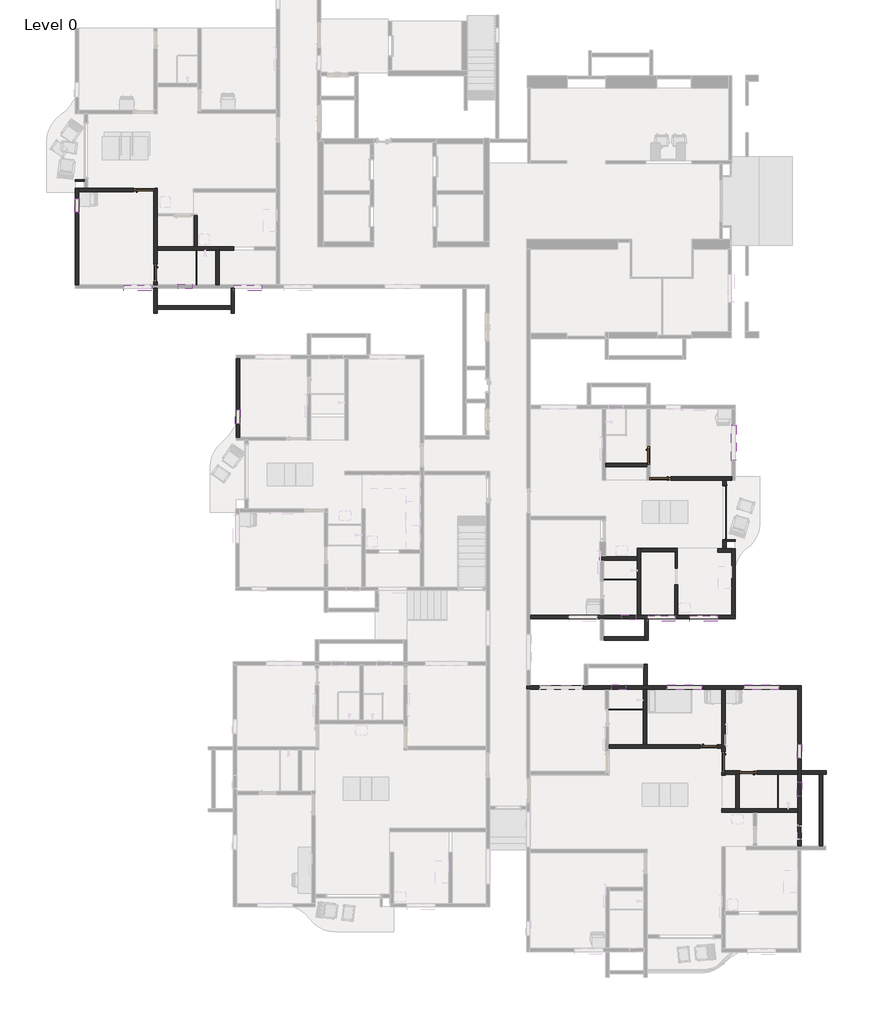
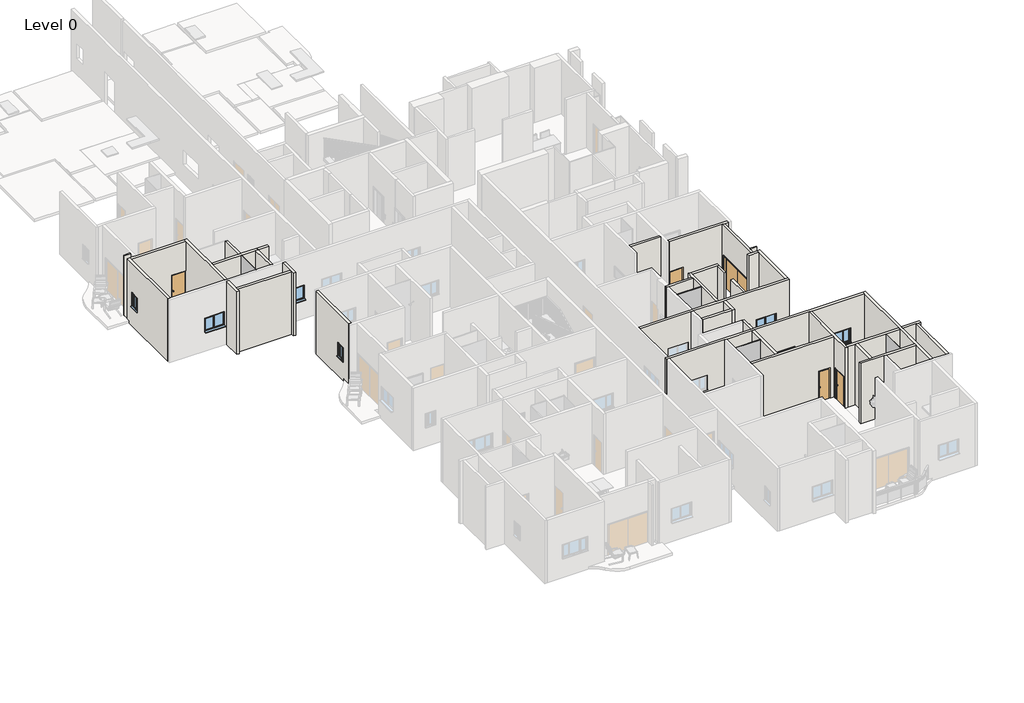
# One storey, part 3 of 14: 35 walls, 14 windows, 8 doors, 4 plates.
"""IFC4 building model written with IfcOpenShell, lengths in millimetres."""

from ifc_helpers import new_model, si_unit, frame, origin, origin_with_axes, place, context, project, spatial, polyline, outline, extrude, faceted_brep, transform, mapped, element, save
from components import doors_concept_intdbl_8_5090a96f, doors_extsgl_flush_d2_fac1298c, doors_extsgl_flush_d2_5e0ff3e2, doors_extsgl_flush_d3_352cde1d, doors_extsgl_flush_d3_ba5ff989, system_panel_glazed_533a1375, system_panel_glazed_d137d5b4, system_panel_glazed_d14c18e3, system_panel_glazed_5123bacf, windows_concept_plain_dbl_4_d1e2e333, windows_sgl_plain_2_be143095, windows_tpl_variable_casement_2_47b04551, windows_tpl_variable_casement_5_ffad3fa3

model = new_model("IFC4")

# Units and contexts
model_context = context("Model", 3, world=origin())
ifc_project = project(units=[si_unit("LENGTHUNIT", "METRE", prefix="MILLI")], contexts=[model_context])

# Site, building, storey
site = spatial("IfcSite", under=ifc_project)
building = spatial("IfcBuilding", under=site)
storey = spatial("IfcBuildingStorey", under=building, Name="Level 0", Elevation=0.0)

# Doors
placement = place(None, origin())
doors_concept_intdbl_8_shape = doors_concept_intdbl_8_5090a96f(model_context)
element("IfcDoor", 1, ObjectType="Doors_Concept_IntDbl : 8'", at=placement, inside=storey, context=model_context, shape_type="MappedRepresentation", body=[
    mapped(doors_concept_intdbl_8_shape, transform((-11246.4933798, 29202.1106683, 0.0), x_axis=(0.0, -1.0, 0.0), y_axis=(1.0, 0.0, 0.0), z_axis=(0.0, 0.0, 1.0))),
])
doors_extsgl_flush_d2_shape = doors_extsgl_flush_d2_fac1298c(model_context)
element("IfcDoor", 2, ObjectType="Doors_ExtSgl_Flush : D2", at=placement, inside=storey, context=model_context, shape_type="MappedRepresentation", body=[
    mapped(doors_extsgl_flush_d2_shape, transform((-11299.3465173, 18242.0106683, 0.0), x_axis=(0.0, -1.0, 0.0), y_axis=(1.0, 0.0, 0.0), z_axis=(0.0, 0.0, 1.0))),
])
doors_extsgl_flush_d2_2_shape = doors_extsgl_flush_d2_5e0ff3e2(model_context)
element("IfcDoor", 3, ObjectType="Doors_ExtSgl_Flush : D2", at=placement, inside=storey, context=model_context, shape_type="MappedRepresentation", body=[
    mapped(doors_extsgl_flush_d2_2_shape, transform((-14088.8486976, 30700.7106683, 0.0), x_axis=(-1.0, 0.0, 0.0), y_axis=(0.0, -1.0, 0.0), z_axis=(0.0, 0.0, 1.0))),
])
element("IfcDoor", 4, ObjectType="Doors_ExtSgl_Flush : D2", at=placement, inside=storey, context=model_context, shape_type="MappedRepresentation", body=[
    mapped(doors_extsgl_flush_d2_2_shape, transform((-36777.1839022, 43403.2998557, 0.0), x_axis=(1.0, 0.0, 0.0), y_axis=(0.0, 1.0, 0.0), z_axis=(0.0, 0.0, 1.0))),
])
doors_extsgl_flush_d3_shape = doors_extsgl_flush_d3_352cde1d(model_context)
element("IfcDoor", 5, ObjectType="Doors_ExtSgl_Flush : D3", at=placement, inside=storey, context=model_context, shape_type="MappedRepresentation", body=[
    mapped(doors_extsgl_flush_d3_shape, transform((-11947.1481173, 18921.5114683, 0.0), x_axis=(1.0, 0.0, 0.0), y_axis=(0.0, 1.0, 0.0), z_axis=(0.0, 0.0, 1.0))),
])
element("IfcDoor", 6, ObjectType="Doors_ExtSgl_Flush : D3", at=placement, inside=storey, context=model_context, shape_type="MappedRepresentation", body=[
    mapped(doors_extsgl_flush_d3_shape, transform((-10211.6953327, 17778.5114683, 0.0), x_axis=(-1.0, 0.0, 0.0), y_axis=(0.0, -1.0, 0.0), z_axis=(0.0, 0.0, 1.0))),
])
element("IfcDoor", 7, ObjectType="Doors_ExtSgl_Flush : D3", at=placement, inside=storey, context=model_context, shape_type="MappedRepresentation", body=[
    mapped(doors_extsgl_flush_d3_shape, transform((-36281.7823022, 39752.8962471, 0.0), x_axis=(0.0, -1.0, 0.0), y_axis=(1.0, 0.0, 0.0), z_axis=(0.0, 0.0, 1.0))),
])
doors_extsgl_flush_d3_2_shape = doors_extsgl_flush_d3_ba5ff989(model_context)
element("IfcDoor", 8, ObjectType="Doors_ExtSgl_Flush : D3", at=placement, inside=storey, context=model_context, shape_type="MappedRepresentation", body=[
    mapped(doors_extsgl_flush_d3_2_shape, transform((-14596.8486976, 31716.7106683, 0.0), x_axis=(0.0, -1.0, 0.0), y_axis=(1.0, 0.0, 0.0), z_axis=(0.0, 0.0, 1.0))),
])

# Plates
system_panel_glazed_shape = system_panel_glazed_533a1375(model_context)
element("IfcPlate", 9, ObjectType="System Panel : Glazed", at=placement, inside=storey, context=model_context, shape_type="MappedRepresentation", body=[
    mapped(system_panel_glazed_shape, transform((-34528.7632652, 39996.9988514, 0.0), x_axis=(0.0, -1.0, 0.0), y_axis=(1.0, 0.0, 0.0), z_axis=(0.0, 0.0, 1.0))),
])
system_panel_glazed_2_shape = system_panel_glazed_d137d5b4(model_context)
element("IfcPlate", 10, ObjectType="System Panel : Glazed", at=placement, inside=storey, context=model_context, shape_type="MappedRepresentation", body=[
    mapped(system_panel_glazed_2_shape, transform((-8932.7419991, 16923.8396258, 0.0), x_axis=(0.0, -1.0, 0.0), y_axis=(1.0, 0.0, 0.0), z_axis=(0.0, 0.0, 1.0))),
])
system_panel_glazed_3_shape = system_panel_glazed_d14c18e3(model_context)
element("IfcPlate", 11, ObjectType="System Panel : Glazed", at=placement, inside=storey, context=model_context, shape_type="MappedRepresentation", body=[
    mapped(system_panel_glazed_3_shape, transform((-15581.2639165, 20578.9122683, 0.0), x_axis=(-1.0, 0.0, 0.0), y_axis=(0.0, -1.0, 0.0), z_axis=(0.0, 0.0, 1.0))),
])
system_panel_glazed_4_shape = system_panel_glazed_5123bacf(model_context)
element("IfcPlate", 12, ObjectType="System Panel : Glazed", at=placement, inside=storey, context=model_context, shape_type="MappedRepresentation", body=[
    mapped(system_panel_glazed_4_shape, transform((-15827.0456172, 26227.359605, 0.0), x_axis=(1.0, 0.0, 0.0), y_axis=(0.0, 1.0, 0.0), z_axis=(0.0, 0.0, 1.0))),
])

# Walls
element("IfcWall", 13, ObjectType="W1", at=placement, inside=storey, context=model_context, shape_type="Brep", body=[
    faceted_brep([(-8039.9933343, 21594.9122683, 0.0), (-8039.9933343, 21442.5122683, 0.0), (-8039.9933343, 17854.7114683, 0.0), (-8039.9933343, 17702.3114683, 0.0), (-8039.9933343, 16175.8530766, 0.0), (-8039.9933343, 16023.4530766, 0.0), (-8039.9933343, 14528.3736639, 0.0), (-8039.9933343, 14528.3736639, 4000.0), (-8039.9933343, 16023.4530766, 4000.0), (-8039.9933343, 16175.8530766, 4000.0), (-8039.9933343, 17702.3114683, 4000.0), (-8039.9933343, 17854.7114683, 4000.0), (-8039.9933343, 21442.5122683, 4000.0), (-8039.9933343, 21594.9122683, 4000.0), (-8039.9933343, 19020.6530766, 2110.0), (-8039.9933343, 18411.0530766, 2110.0), (-8039.9933343, 18411.0530766, 1200.0), (-8039.9933343, 19020.6530766, 1200.0), (-8039.9933343, 15442.7736639, 2738.9328), (-8039.9933343, 14833.1736639, 2738.9328), (-8039.9933343, 14833.1736639, 1828.9328), (-8039.9933343, 15442.7736639, 1828.9328), (-8039.9933343, 17344.2530766, 2738.9328), (-8039.9933343, 16734.6530766, 2738.9328), (-8039.9933343, 16734.6530766, 1828.9328), (-8039.9933343, 17344.2530766, 1828.9328), (-7887.5933343, 21594.9122683, 0.0), (-7887.5933343, 21594.9122683, 4000.0), (-7887.5933343, 17854.7114683, 4000.0), (-7887.5933343, 17702.3114683, 4000.0), (-7887.5933343, 14528.3736639, 4000.0), (-7887.5933343, 14528.3736639, 0.0), (-7887.5933343, 17702.3114683, 0.0), (-7887.5933343, 17854.7114683, 0.0), (-7887.5933343, 19020.6530766, 2110.0), (-7887.5933343, 19020.6530766, 1200.0), (-7887.5933343, 18411.0530766, 1200.0), (-7887.5933343, 18411.0530766, 2110.0), (-7887.5933343, 15442.7736639, 2738.9328), (-7887.5933343, 15442.7736639, 1828.9328), (-7887.5933343, 14833.1736639, 1828.9328), (-7887.5933343, 14833.1736639, 2738.9328), (-7887.5933343, 17344.2530766, 2738.9328), (-7887.5933343, 17344.2530766, 1828.9328), (-7887.5933343, 16734.6530766, 1828.9328), (-7887.5933343, 16734.6530766, 2738.9328)], [[[0, 1, 2, 3, 4, 5, 6, 7, 8, 9, 10, 11, 12, 13], [14, 15, 16, 17], [18, 19, 20, 21], [22, 23, 24, 25]], [[26, 27, 28, 29, 30, 31, 32, 33], [34, 35, 36, 37], [38, 39, 40, 41], [42, 43, 44, 45]], [[6, 5, 4, 3, 2, 1, 0, 26, 33, 32, 31]], [[13, 12, 11, 10, 9, 8, 7, 30, 29, 28, 27]], [[7, 6, 31, 30]], [[0, 13, 27, 26]], [[35, 34, 14, 17]], [[36, 35, 17, 16]], [[37, 36, 16, 15]], [[34, 37, 15, 14]], [[39, 38, 18, 21]], [[40, 39, 21, 20]], [[41, 40, 20, 19]], [[38, 41, 19, 18]], [[43, 42, 22, 25]], [[44, 43, 25, 24]], [[45, 44, 24, 23]], [[42, 45, 23, 22]]]),
])
element("IfcWall", 14, ObjectType="W1", at=placement, inside=storey, context=model_context, shape_type="Brep", body=[
    faceted_brep([(-8039.9933343, 21594.9122683, 0.0), (-14657.7537173, 21594.9122683, 0.0), (-14810.1537173, 21594.9122683, 0.0), (-17277.7094141, 21594.9122683, 0.0), (-17430.1094141, 21594.9122683, 0.0), (-19793.4917798, 21594.9122683, 0.0), (-19945.8917798, 21594.9122683, 0.0), (-19965.3949343, 21594.9122683, 0.0), (-19965.3949343, 21594.9122683, 4000.0), (-19945.8917798, 21594.9122683, 4000.0), (-19793.4917798, 21594.9122683, 4000.0), (-17430.1094141, 21594.9122683, 4000.0), (-17277.7094141, 21594.9122683, 4000.0), (-14810.1537173, 21594.9122683, 4000.0), (-14657.7537173, 21594.9122683, 4000.0), (-8039.9933343, 21594.9122683, 4000.0), (-19360.5094141, 21594.9122683, 2110.0), (-19360.5094141, 21594.9122683, 1200.0), (-17531.7094141, 21594.9122683, 1200.0), (-17531.7094141, 21594.9122683, 2110.0), (-13778.6501173, 21594.9122683, 2110.0), (-13778.6501173, 21594.9122683, 1200.0), (-12254.6501173, 21594.9122683, 1200.0), (-12254.6501173, 21594.9122683, 2110.0), (-10393.5699258, 21594.9122683, 2110.0), (-10393.5699258, 21594.9122683, 1200.0), (-8869.5699258, 21594.9122683, 1200.0), (-8869.5699258, 21594.9122683, 2110.0), (-16212.6741157, 21594.9122683, 2738.9328), (-16212.6741157, 21594.9122683, 1828.9328), (-15603.0741157, 21594.9122683, 1828.9328), (-15603.0741157, 21594.9122683, 2738.9328), (-8039.9933343, 21442.5122683, 0.0), (-8039.9933343, 21442.5122683, 4000.0), (-11223.1465173, 21442.5122683, 4000.0), (-11375.5465173, 21442.5122683, 4000.0), (-14670.4537173, 21442.5122683, 4000.0), (-14822.8537173, 21442.5122683, 4000.0), (-16339.6741157, 21442.5122683, 4000.0), (-16492.0741157, 21442.5122683, 4000.0), (-19812.9949343, 21442.5122683, 4000.0), (-19965.3949343, 21442.5122683, 4000.0), (-19965.3949343, 21442.5122683, 0.0), (-19812.9949343, 21442.5122683, 0.0), (-16492.0741157, 21442.5122683, 0.0), (-16339.6741157, 21442.5122683, 0.0), (-14822.8537173, 21442.5122683, 0.0), (-14670.4537173, 21442.5122683, 0.0), (-11375.5465173, 21442.5122683, 0.0), (-11223.1465173, 21442.5122683, 0.0), (-19360.5094141, 21442.5122683, 2110.0), (-17531.7094141, 21442.5122683, 2110.0), (-17531.7094141, 21442.5122683, 1200.0), (-19360.5094141, 21442.5122683, 1200.0), (-13778.6501173, 21442.5122683, 2110.0), (-12254.6501173, 21442.5122683, 2110.0), (-12254.6501173, 21442.5122683, 1200.0), (-13778.6501173, 21442.5122683, 1200.0), (-10393.5699258, 21442.5122683, 2110.0), (-8869.5699258, 21442.5122683, 2110.0), (-8869.5699258, 21442.5122683, 1200.0), (-10393.5699258, 21442.5122683, 1200.0), (-16212.6741157, 21442.5122683, 2738.9328), (-15603.0741157, 21442.5122683, 2738.9328), (-15603.0741157, 21442.5122683, 1828.9328), (-16212.6741157, 21442.5122683, 1828.9328)], [[[0, 1, 2, 3, 4, 5, 6, 7, 8, 9, 10, 11, 12, 13, 14, 15], [16, 17, 18, 19], [20, 21, 22, 23], [24, 25, 26, 27], [28, 29, 30, 31]], [[32, 33, 34, 35, 36, 37, 38, 39, 40, 41, 42, 43, 44, 45, 46, 47, 48, 49], [50, 51, 52, 53], [54, 55, 56, 57], [58, 59, 60, 61], [62, 63, 64, 65]], [[7, 6, 5, 4, 3, 2, 1, 0, 32, 49, 48, 47, 46, 45, 44, 43, 42]], [[15, 14, 13, 12, 11, 10, 9, 8, 41, 40, 39, 38, 37, 36, 35, 34, 33]], [[0, 15, 33, 32]], [[8, 7, 42, 41]], [[17, 16, 50, 53]], [[18, 17, 53, 52]], [[19, 18, 52, 51]], [[16, 19, 51, 50]], [[21, 20, 54, 57]], [[22, 21, 57, 56]], [[23, 22, 56, 55]], [[20, 23, 55, 54]], [[25, 24, 58, 61]], [[26, 25, 61, 60]], [[27, 26, 60, 59]], [[24, 27, 59, 58]], [[29, 28, 62, 65]], [[30, 29, 65, 64]], [[31, 30, 64, 63]], [[28, 31, 63, 62]]]),
])
element("IfcWall", 15, ObjectType="W1", at=placement, inside=storey, context=model_context, shape_type="Brep", body=[
    faceted_brep([(-11566.1481173, 18845.3114683, 2110.0), (-11566.1481173, 18845.3114683, 0.0), (-11375.5465173, 18845.3114683, 0.0), (-11375.5465173, 18845.3114683, 4000.0), (-16339.6741157, 18845.3114683, 4000.0), (-16339.6741157, 18845.3114683, 0.0), (-12328.1481173, 18845.3114683, 0.0), (-12328.1481173, 18845.3114683, 2110.0), (-11375.5465173, 18997.7114683, 0.0), (-11566.1481173, 18997.7114683, 0.0), (-11566.1481173, 18997.7114683, 2110.0), (-12328.1481173, 18997.7114683, 2110.0), (-12328.1481173, 18997.7114683, 0.0), (-14670.4537173, 18997.7114683, 0.0), (-14822.8537173, 18997.7114683, 0.0), (-16339.6741157, 18997.7114683, 0.0), (-16339.6741157, 18997.7114683, 4000.0), (-14822.8537173, 18997.7114683, 4000.0), (-14670.4537173, 18997.7114683, 4000.0), (-11375.5465173, 18997.7114683, 4000.0)], [[[0, 1, 2, 3, 4, 5, 6, 7]], [[8, 9, 10, 11, 12, 13, 14, 15, 16, 17, 18, 19]], [[6, 5, 15, 14, 13, 12]], [[2, 1, 9, 8]], [[4, 3, 19, 18, 17, 16]], [[5, 4, 16, 15]], [[3, 2, 8, 19]], [[12, 11, 7, 6]], [[10, 9, 1, 0]], [[11, 10, 0, 7]]]),
])
element("IfcWall", 16, ObjectType="W1", at=placement, inside=storey, context=model_context, shape_type="SweptSolid", body=[
    extrude(outline(polyline([(-14822.8537173, 18997.7114683), (-14822.8537173, 21442.5122683), (-14670.4537173, 21442.5122683), (-14670.4537173, 18997.7114683), (-14822.8537173, 18997.7114683)])), origin_with_axes(), (0.0, 0.0, 1.0), 4000.0),
])
element("IfcWall", 17, ObjectType="W1", at=placement, inside=storey, context=model_context, shape_type="Brep", body=[
    faceted_brep([(-11375.5465173, 17784.8106683, 2110.0), (-11375.5465173, 17784.8106683, 0.0), (-11375.5465173, 17651.5114683, 0.0), (-11375.5465173, 17651.5114683, 4000.0), (-11375.5465173, 18845.3114683, 4000.0), (-11375.5465173, 18997.7114683, 4000.0), (-11375.5465173, 21442.5122683, 4000.0), (-11375.5465173, 21442.5122683, 0.0), (-11375.5465173, 18997.7114683, 0.0), (-11375.5465173, 18845.3114683, 0.0), (-11375.5465173, 18699.2106683, 0.0), (-11375.5465173, 18699.2106683, 2110.0), (-11223.1465173, 17651.5114683, 0.0), (-11223.1465173, 17702.3114683, 0.0), (-11223.1465173, 17784.8106683, 0.0), (-11223.1465173, 17784.8106683, 2110.0), (-11223.1465173, 18699.2106683, 2110.0), (-11223.1465173, 18699.2106683, 0.0), (-11223.1465173, 21442.5122683, 0.0), (-11223.1465173, 21442.5122683, 4000.0), (-11223.1465173, 17854.7114683, 4000.0), (-11223.1465173, 17702.3114683, 4000.0), (-11223.1465173, 17651.5114683, 4000.0)], [[[0, 1, 2, 3, 4, 5, 6, 7, 8, 9, 10, 11]], [[12, 13, 14, 15, 16, 17, 18, 19, 20, 21, 22]], [[2, 1, 14, 13, 12]], [[10, 9, 8, 7, 18, 17]], [[3, 2, 12, 22]], [[6, 5, 4, 3, 22, 21, 20, 19]], [[7, 6, 19, 18]], [[17, 16, 11, 10]], [[15, 14, 1, 0]], [[16, 15, 0, 11]]]),
])
element("IfcWall", 18, ObjectType="W1", at=placement, inside=storey, context=model_context, shape_type="Brep", body=[
    faceted_brep([(-6784.5473173, 17702.3114683, 0.0), (-6784.5473173, 17702.3114683, 4000.0), (-6936.9473173, 17702.3114683, 4000.0), (-7089.3473173, 17702.3114683, 4000.0), (-7887.5933343, 17702.3114683, 4000.0), (-7887.5933343, 17702.3114683, 0.0), (-7089.3473173, 17702.3114683, 0.0), (-6936.9473173, 17702.3114683, 0.0), (-6784.5473173, 17854.7114683, 4000.0), (-6784.5473173, 17854.7114683, 0.0), (-7887.5933343, 17854.7114683, 0.0), (-7887.5933343, 17854.7114683, 4000.0)], [[[0, 1, 2, 3, 4, 5, 6, 7]], [[8, 9, 10, 11]], [[9, 0, 7, 6, 5, 10]], [[1, 0, 9, 8]], [[1, 8, 11, 4, 3, 2]], [[5, 4, 11, 10]]]),
    faceted_brep([(-11223.1465173, 17702.3114683, 4000.0), (-11223.1465173, 17702.3114683, 0.0), (-10757.7953327, 17702.3114683, 0.0), (-10605.3953327, 17702.3114683, 0.0), (-10592.6953327, 17702.3114683, 0.0), (-10592.6953327, 17702.3114683, 2110.0), (-9830.6953327, 17702.3114683, 2110.0), (-9830.6953327, 17702.3114683, 0.0), (-8039.9933343, 17702.3114683, 0.0), (-8039.9933343, 17702.3114683, 4000.0), (-10605.3953327, 17702.3114683, 4000.0), (-10757.7953327, 17702.3114683, 4000.0), (-11223.1465173, 17854.7114683, 0.0), (-11223.1465173, 17854.7114683, 4000.0), (-8039.9933343, 17854.7114683, 4000.0), (-8039.9933343, 17854.7114683, 0.0), (-9830.6953327, 17854.7114683, 0.0), (-9830.6953327, 17854.7114683, 2110.0), (-10592.6953327, 17854.7114683, 2110.0), (-10592.6953327, 17854.7114683, 0.0), (-11223.1465173, 17784.8106683, 0.0)], [[[0, 1, 2, 3, 4, 5, 6, 7, 8, 9, 10, 11]], [[12, 13, 14, 15, 16, 17, 18, 19]], [[1, 20, 12, 19, 4, 3, 2]], [[7, 16, 15, 8]], [[13, 0, 11, 10, 9, 14]], [[1, 0, 13, 12, 20]], [[9, 8, 15, 14]], [[7, 6, 17, 16]], [[5, 4, 19, 18]], [[6, 5, 18, 17]]]),
])
element("IfcWall", 19, ObjectType="W1", at=placement, inside=storey, context=model_context, shape_type="Brep", body=[
    faceted_brep([(-11385.349671, 16023.4530766, 0.0), (-9995.7953327, 16023.4530766, 0.0), (-9843.3953327, 16023.4530766, 0.0), (-8039.9933343, 16023.4530766, 0.0), (-8039.9933343, 16023.4530766, 4000.0), (-9843.3953327, 16023.4530766, 4000.0), (-9995.7953327, 16023.4530766, 4000.0), (-11385.349671, 16023.4530766, 4000.0), (-11385.349671, 16175.8530766, 0.0), (-11385.349671, 16175.8530766, 4000.0), (-10757.7953327, 16175.8530766, 4000.0), (-10605.3953327, 16175.8530766, 4000.0), (-8039.9933343, 16175.8530766, 4000.0), (-8039.9933343, 16175.8530766, 0.0), (-10605.3953327, 16175.8530766, 0.0), (-10757.7953327, 16175.8530766, 0.0)], [[[0, 1, 2, 3, 4, 5, 6, 7]], [[8, 9, 10, 11, 12, 13, 14, 15]], [[3, 2, 1, 0, 8, 15, 14, 13]], [[7, 6, 5, 4, 12, 11, 10, 9]], [[0, 7, 9, 8]], [[4, 3, 13, 12]]]),
])
element("IfcWall", 20, ObjectType="W1", at=placement, inside=storey, context=model_context, shape_type="SweptSolid", body=[
    extrude(outline(polyline([(-10757.7953327, 16175.8530766), (-10757.7953327, 17702.3114683), (-10605.3953327, 17702.3114683), (-10605.3953327, 16175.8530766), (-10757.7953327, 16175.8530766)])), origin_with_axes(), (0.0, 0.0, 1.0), 4000.0),
])
element("IfcWall", 21, ObjectType="W1", at=placement, inside=storey, context=model_context, shape_type="SweptSolid", body=[
    extrude(outline(polyline([(35984.9800488, 0.0), (32534.4541094, 0.0), (32534.4541094, 4000.0), (35984.9800488, 4000.0), (35984.9800488, 0.0)]), holes=[polyline([(33118.6541094, 2110.0), (33118.6541094, 1200.0), (33728.2541094, 1200.0), (33728.2541094, 2110.0), (33118.6541094, 2110.0)])]), frame((-32744.0041796, 0.0, 0.0), z_axis=(1.0, 0.0, 0.0), x_axis=(0.0, 1.0, 0.0)), (0.0, 0.0, 1.0), 152.4),
])
element("IfcWall", 22, ObjectType="W1", at=placement, inside=storey, context=model_context, shape_type="Brep", body=[
    faceted_brep([(-14657.7537173, 21594.9122683, 0.0), (-14657.7537173, 22534.7122683, 0.0), (-14657.7537173, 22534.7122683, 4000.0), (-14657.7537173, 21594.9122683, 4000.0), (-14810.1537173, 21594.9122683, 0.0), (-14810.1537173, 21594.9122683, 4000.0), (-14810.1537173, 22382.3122683, 4000.0), (-14810.1537173, 22534.7122683, 4000.0), (-14810.1537173, 22534.7122683, 0.0), (-14810.1537173, 22382.3122683, 0.0)], [[[0, 1, 2, 3]], [[4, 5, 6, 7, 8, 9]], [[1, 0, 4, 9, 8]], [[3, 2, 7, 6, 5]], [[0, 3, 5, 4]], [[2, 1, 8, 7]]]),
])
element("IfcWall", 23, ObjectType="W1", at=placement, inside=storey, context=model_context, shape_type="Brep", body=[
    faceted_brep([(-19793.4917798, 24541.3122683, 0.0), (-16716.0456172, 24541.3122683, 0.0), (-16563.6456172, 24541.3122683, 0.0), (-14760.1440172, 24541.3122683, 0.0), (-14607.7440172, 24541.3122683, 0.0), (-10776.4917798, 24541.3122683, 0.0), (-10776.4917798, 24541.3122683, 4000.0), (-14607.7440172, 24541.3122683, 4000.0), (-14760.1440172, 24541.3122683, 4000.0), (-16563.6456172, 24541.3122683, 4000.0), (-16716.0456172, 24541.3122683, 4000.0), (-19793.4917798, 24541.3122683, 4000.0), (-16872.4917798, 24541.3122683, 2110.0), (-16872.4917798, 24541.3122683, 1200.0), (-18091.6917798, 24541.3122683, 1200.0), (-18091.6917798, 24541.3122683, 2110.0), (-13414.0456172, 24541.3122683, 2110.0), (-13414.0456172, 24541.3122683, 1200.0), (-14633.2456172, 24541.3122683, 1200.0), (-14633.2456172, 24541.3122683, 2110.0), (-11561.8686985, 24541.3122683, 2110.0), (-11561.8686985, 24541.3122683, 1200.0), (-12781.0686985, 24541.3122683, 1200.0), (-12781.0686985, 24541.3122683, 2110.0), (-15166.6456172, 24541.3122683, 2738.9328), (-15166.6456172, 24541.3122683, 1828.9328), (-15776.2456172, 24541.3122683, 1828.9328), (-15776.2456172, 24541.3122683, 2738.9328), (-19793.4917798, 24693.7122683, 0.0), (-19793.4917798, 24693.7122683, 4000.0), (-16716.0456172, 24693.7122683, 4000.0), (-16563.6456172, 24693.7122683, 4000.0), (-15090.4456172, 24693.7122683, 4000.0), (-14938.0456172, 24693.7122683, 4000.0), (-13439.3440172, 24693.7122683, 4000.0), (-13312.2424172, 24693.7122683, 4000.0), (-10928.8917798, 24693.7122683, 4000.0), (-10776.4917798, 24693.7122683, 4000.0), (-10776.4917798, 24693.7122683, 0.0), (-10928.8917798, 24693.7122683, 0.0), (-13312.2424172, 24693.7122683, 0.0), (-13439.3440172, 24693.7122683, 0.0), (-14938.0456172, 24693.7122683, 0.0), (-15090.4456172, 24693.7122683, 0.0), (-16563.6456172, 24693.7122683, 0.0), (-16716.0456172, 24693.7122683, 0.0), (-16872.4917798, 24693.7122683, 2110.0), (-18091.6917798, 24693.7122683, 2110.0), (-18091.6917798, 24693.7122683, 1200.0), (-16872.4917798, 24693.7122683, 1200.0), (-13414.0456172, 24693.7122683, 2110.0), (-14633.2456172, 24693.7122683, 2110.0), (-14633.2456172, 24693.7122683, 1200.0), (-13414.0456172, 24693.7122683, 1200.0), (-11561.8686985, 24693.7122683, 2110.0), (-12781.0686985, 24693.7122683, 2110.0), (-12781.0686985, 24693.7122683, 1200.0), (-11561.8686985, 24693.7122683, 1200.0), (-15166.6456172, 24693.7122683, 2738.9328), (-15776.2456172, 24693.7122683, 2738.9328), (-15776.2456172, 24693.7122683, 1828.9328), (-15166.6456172, 24693.7122683, 1828.9328)], [[[0, 1, 2, 3, 4, 5, 6, 7, 8, 9, 10, 11], [12, 13, 14, 15], [16, 17, 18, 19], [20, 21, 22, 23], [24, 25, 26, 27]], [[28, 29, 30, 31, 32, 33, 34, 35, 36, 37, 38, 39, 40, 41, 42, 43, 44, 45], [46, 47, 48, 49], [50, 51, 52, 53], [54, 55, 56, 57], [58, 59, 60, 61]], [[5, 4, 3, 2, 1, 0, 28, 45, 44, 43, 42, 41, 40, 39, 38]], [[11, 10, 9, 8, 7, 6, 37, 36, 35, 34, 33, 32, 31, 30, 29]], [[0, 11, 29, 28]], [[6, 5, 38, 37]], [[13, 12, 46, 49]], [[14, 13, 49, 48]], [[15, 14, 48, 47]], [[12, 15, 47, 46]], [[17, 16, 50, 53]], [[18, 17, 53, 52]], [[19, 18, 52, 51]], [[16, 19, 51, 50]], [[21, 20, 54, 57]], [[22, 21, 57, 56]], [[23, 22, 56, 55]], [[20, 23, 55, 54]], [[25, 24, 58, 61]], [[26, 25, 61, 60]], [[27, 26, 60, 59]], [[24, 27, 59, 58]]]),
])
element("IfcWall", 24, ObjectType="W1", at=placement, inside=storey, context=model_context, shape_type="Brep", body=[
    faceted_brep([(-14938.0456172, 24693.7122683, 0.0), (-14938.0456172, 27487.7122683, 0.0), (-14938.0456172, 27640.1122683, 0.0), (-14938.0456172, 27640.1122683, 4000.0), (-14938.0456172, 27487.7122683, 4000.0), (-14938.0456172, 24693.7122683, 4000.0), (-15090.4456172, 24693.7122683, 0.0), (-15090.4456172, 24693.7122683, 4000.0), (-15090.4456172, 27104.561205, 4000.0), (-15090.4456172, 27256.961205, 4000.0), (-15090.4456172, 27640.1122683, 4000.0), (-15090.4456172, 27640.1122683, 0.0), (-15090.4456172, 27256.961205, 0.0), (-15090.4456172, 27104.561205, 0.0)], [[[0, 1, 2, 3, 4, 5]], [[6, 7, 8, 9, 10, 11, 12, 13]], [[2, 1, 0, 6, 13, 12, 11]], [[5, 4, 3, 10, 9, 8, 7]], [[0, 5, 7, 6]], [[3, 2, 11, 10]]]),
])
element("IfcWall", 25, ObjectType="W1", at=placement, inside=storey, context=model_context, shape_type="Brep", body=[
    faceted_brep([(-15090.4456172, 27256.961205, 0.0), (-16484.7370231, 27256.961205, 0.0), (-16745.0362231, 27256.961205, 0.0), (-16745.0362231, 27256.961205, 4000.0), (-16484.7370231, 27256.961205, 4000.0), (-15090.4456172, 27256.961205, 4000.0), (-15090.4456172, 27104.561205, 0.0), (-15090.4456172, 27104.561205, 4000.0), (-16563.6456172, 27104.561205, 4000.0), (-16716.0456172, 27104.561205, 4000.0), (-16745.0362231, 27104.561205, 4000.0), (-16745.0362231, 27104.561205, 0.0), (-16716.0456172, 27104.561205, 0.0), (-16563.6456172, 27104.561205, 0.0)], [[[0, 1, 2, 3, 4, 5]], [[6, 7, 8, 9, 10, 11, 12, 13]], [[2, 1, 0, 6, 13, 12, 11]], [[5, 4, 3, 10, 9, 8, 7]], [[0, 5, 7, 6]], [[3, 2, 11, 10]]]),
])
element("IfcWall", 26, ObjectType="W1", at=placement, inside=storey, context=model_context, shape_type="SweptSolid", body=[
    extrude(outline(polyline([(-14673.0486976, 31234.1106683), (-16476.4486976, 31234.1106683), (-16476.4486976, 31386.5106683), (-14673.0486976, 31386.5106683), (-14673.0486976, 31234.1106683)])), origin_with_axes(), (0.0, 0.0, 1.0), 4000.0),
])
element("IfcWall", 27, ObjectType="W1", at=placement, inside=storey, context=model_context, shape_type="Brep", body=[
    faceted_brep([(-14520.6486976, 30776.9106683, 4000.0), (-10935.2417798, 30776.9106683, 4000.0), (-10935.2417798, 30776.9106683, 0.0), (-13631.6486976, 30776.9106683, 0.0), (-13631.6486976, 30776.9106683, 2110.0), (-14520.6486976, 30776.9106683, 2110.0), (-10935.2417798, 30624.5106683, 4000.0), (-11170.2933798, 30624.5106683, 4000.0), (-11322.6933798, 30624.5106683, 4000.0), (-14520.6486976, 30624.5106683, 4000.0), (-14520.6486976, 30624.5106683, 2110.0), (-13631.6486976, 30624.5106683, 2110.0), (-13631.6486976, 30624.5106683, 0.0), (-11322.6933798, 30624.5106683, 0.0), (-11170.2933798, 30624.5106683, 0.0), (-10935.2417798, 30624.5106683, 0.0)], [[[0, 1, 2, 3, 4, 5]], [[6, 7, 8, 9, 10, 11, 12, 13, 14, 15]], [[2, 15, 14, 13, 12, 3]], [[1, 0, 9, 8, 7, 6]], [[9, 0, 5, 10]], [[2, 1, 6, 15]], [[11, 4, 3, 12]], [[4, 11, 10, 5]]]),
])
element("IfcWall", 28, ObjectType="W1", at=placement, inside=storey, context=model_context, shape_type="Brep", body=[
    faceted_brep([(-14938.0456172, 27487.7122683, 0.0), (-13413.8932172, 27487.7122683, 0.0), (-13344.0940172, 27487.7122683, 0.0), (-13344.0940172, 27487.7122683, 4000.0), (-13413.8932172, 27487.7122683, 4000.0), (-14938.0456172, 27487.7122683, 4000.0), (-14938.0456172, 27640.1122683, 0.0), (-14938.0456172, 27640.1122683, 4000.0), (-13344.0940172, 27640.1122683, 4000.0), (-13344.0940172, 27640.1122683, 0.0)], [[[0, 1, 2, 3, 4, 5]], [[6, 7, 8, 9]], [[2, 1, 0, 6, 9]], [[5, 4, 3, 8, 7]], [[0, 5, 7, 6]], [[3, 2, 9, 8]]]),
])
element("IfcWall", 29, ObjectType="W1", at=placement, inside=storey, context=model_context, shape_type="Brep", body=[
    faceted_brep([(-10776.4917798, 24693.7122683, 0.0), (-10776.4917798, 27614.7122683, 0.0), (-10776.4917798, 27614.7122683, 4000.0), (-10776.4917798, 24693.7122683, 4000.0), (-10928.8917798, 24693.7122683, 0.0), (-10928.8917798, 24693.7122683, 4000.0), (-10928.8917798, 27462.3122683, 4000.0), (-10928.8917798, 27614.7122683, 4000.0), (-10928.8917798, 27614.7122683, 0.0), (-10928.8917798, 27462.3122683, 0.0)], [[[0, 1, 2, 3]], [[4, 5, 6, 7, 8, 9]], [[1, 0, 4, 9, 8]], [[3, 2, 7, 6, 5]], [[0, 3, 5, 4]], [[2, 1, 8, 7]]]),
])
element("IfcWall", 30, ObjectType="W1", at=placement, inside=storey, context=model_context, shape_type="Brep", body=[
    faceted_brep([(-10928.8917798, 27614.7122683, 0.0), (-11170.2933798, 27614.7122683, 0.0), (-11322.6933798, 27614.7122683, 0.0), (-11551.2933798, 27614.7122683, 0.0), (-11551.2933798, 27614.7122683, 4000.0), (-11322.6933798, 27614.7122683, 4000.0), (-11170.2933798, 27614.7122683, 4000.0), (-10928.8917798, 27614.7122683, 4000.0), (-10928.8917798, 27462.3122683, 0.0), (-10928.8917798, 27462.3122683, 4000.0), (-11551.2933798, 27462.3122683, 4000.0), (-11551.2933798, 27462.3122683, 0.0)], [[[0, 1, 2, 3, 4, 5, 6, 7]], [[8, 9, 10, 11]], [[3, 2, 1, 0, 8, 11]], [[4, 3, 11, 10]], [[7, 6, 5, 4, 10, 9]], [[0, 7, 9, 8]]]),
])
element("IfcWall", 31, ObjectType="W1", at=placement, inside=storey, context=model_context, shape_type="Brep", body=[
    faceted_brep([(-11170.2933798, 30624.5106683, 4000.0), (-11170.2933798, 28008.4122683, 4000.0), (-11170.2933798, 27938.6130683, 4000.0), (-11170.2933798, 27614.7122683, 4000.0), (-11170.2933798, 27614.7122683, 0.0), (-11170.2933798, 27938.6130683, 0.0), (-11170.2933798, 27982.9106683, 0.0), (-11170.2933798, 27982.9106683, 2110.0), (-11170.2933798, 30421.3106683, 2110.0), (-11170.2933798, 30421.3106683, 0.0), (-11170.2933798, 30624.5106683, 0.0), (-11322.6933798, 27614.7122683, 4000.0), (-11322.6933798, 30624.5106683, 4000.0), (-11322.6933798, 30624.5106683, 0.0), (-11322.6933798, 30421.3106683, 0.0), (-11322.6933798, 30421.3106683, 2110.0), (-11322.6933798, 27982.9106683, 2110.0), (-11322.6933798, 27982.9106683, 0.0), (-11322.6933798, 27614.7122683, 0.0)], [[[0, 1, 2, 3, 4, 5, 6, 7, 8, 9, 10]], [[11, 12, 13, 14, 15, 16, 17, 18]], [[4, 18, 17, 6, 5]], [[13, 10, 9, 14]], [[3, 2, 1, 0, 12, 11]], [[0, 10, 13, 12]], [[4, 3, 11, 18]], [[16, 7, 6, 17]], [[7, 16, 15, 8]], [[8, 15, 14, 9]]]),
])
element("IfcWall", 32, ObjectType="W1", at=placement, inside=storey, context=model_context, shape_type="Brep", body=[
    faceted_brep([(-14760.1440172, 24541.3122683, 0.0), (-14760.1440172, 23745.411205, 0.0), (-14760.1440172, 23593.011205, 0.0), (-14760.1440172, 23588.7106683, 0.0), (-14760.1440172, 23588.7106683, 4000.0), (-14760.1440172, 23593.011205, 4000.0), (-14760.1440172, 23745.411205, 4000.0), (-14760.1440172, 24541.3122683, 4000.0), (-14607.7440172, 24541.3122683, 0.0), (-14607.7440172, 24541.3122683, 4000.0), (-14607.7440172, 23588.7106683, 4000.0), (-14607.7440172, 23588.7106683, 0.0)], [[[0, 1, 2, 3, 4, 5, 6, 7]], [[8, 9, 10, 11]], [[3, 2, 1, 0, 8, 11]], [[4, 3, 11, 10]], [[7, 6, 5, 4, 10, 9]], [[0, 7, 9, 8]]]),
])
element("IfcWall", 33, ObjectType="W1", at=placement, inside=storey, context=model_context, shape_type="Brep", body=[
    faceted_brep([(-32965.5816447, 39085.2998557, 0.0), (-32965.5816447, 38297.8998557, 0.0), (-32965.5816447, 38145.4998557, 0.0), (-32965.5816447, 37980.2982557, 0.0), (-32965.5816447, 37980.2982557, 4000.0), (-32965.5816447, 38145.4998557, 4000.0), (-32965.5816447, 38297.8998557, 4000.0), (-32965.5816447, 39085.2998557, 4000.0), (-32813.1816447, 39085.2998557, 0.0), (-32813.1816447, 39085.2998557, 4000.0), (-32813.1816447, 37980.2982557, 4000.0), (-32813.1816447, 37980.2982557, 0.0)], [[[0, 1, 2, 3, 4, 5, 6, 7]], [[8, 9, 10, 11]], [[3, 2, 1, 0, 8, 11]], [[4, 3, 11, 10]], [[7, 6, 5, 4, 10, 9]], [[0, 7, 9, 8]]]),
])
element("IfcWall", 34, ObjectType="W1", at=placement, inside=storey, context=model_context, shape_type="Brep", body=[
    faceted_brep([(-36357.9823022, 37987.6978471, 0.0), (-36357.9823022, 37987.6978471, 4000.0), (-36357.9823022, 39085.2998557, 4000.0), (-36357.9823022, 39085.2998557, 0.0), (-36205.5823022, 37987.6978471, 4000.0), (-36205.5823022, 37987.6978471, 0.0), (-36205.5823022, 38145.4998557, 0.0), (-36205.5823022, 38297.8998557, 0.0), (-36205.5823022, 39085.2998557, 0.0), (-36205.5823022, 39085.2998557, 4000.0), (-36205.5823022, 38297.8998557, 4000.0), (-36205.5823022, 38145.4998557, 4000.0)], [[[0, 1, 2, 3]], [[4, 5, 6, 7, 8, 9, 10, 11]], [[5, 0, 3, 8, 7, 6]], [[1, 0, 5, 4]], [[1, 4, 11, 10, 9, 2]], [[3, 2, 9, 8]]]),
    faceted_brep([(-36357.9823022, 43479.4998557, 4000.0), (-36357.9823022, 43479.4998557, 2110.0), (-36357.9823022, 43327.0998557, 2110.0), (-36357.9823022, 43327.0998557, 0.0), (-36357.9823022, 40133.8962471, 0.0), (-36357.9823022, 40133.8962471, 2110.0), (-36357.9823022, 39371.8962471, 2110.0), (-36357.9823022, 39371.8962471, 0.0), (-36357.9823022, 39237.6998557, 0.0), (-36357.9823022, 39237.6998557, 4000.0), (-36357.9823022, 43327.0998557, 4000.0), (-36205.5823022, 43479.4998557, 0.0), (-36205.5823022, 43479.4998557, 4000.0), (-36205.5823022, 42343.7978471, 4000.0), (-36205.5823022, 42273.9986471, 4000.0), (-36205.5823022, 40908.6978471, 4000.0), (-36205.5823022, 40756.2978471, 4000.0), (-36205.5823022, 39237.6998557, 4000.0), (-36205.5823022, 39237.6998557, 0.0), (-36205.5823022, 39371.8962471, 0.0), (-36205.5823022, 39371.8962471, 2110.0), (-36205.5823022, 40133.8962471, 2110.0), (-36205.5823022, 40133.8962471, 0.0), (-36205.5823022, 40756.2978471, 0.0), (-36205.5823022, 40908.6978471, 0.0), (-36205.5823022, 42273.9986471, 0.0), (-36205.5823022, 42343.7978471, 0.0), (-36319.9839022, 43479.4998557, 0.0), (-36319.9839022, 43327.0998557, 0.0), (-36319.9839022, 43479.4998557, 2110.0), (-36319.9839022, 43327.0998557, 2110.0)], [[[0, 1, 2, 3, 4, 5, 6, 7, 8, 9, 10]], [[11, 12, 13, 14, 15, 16, 17, 18, 19, 20, 21, 22, 23, 24, 25, 26]], [[27, 11, 26, 25, 24, 23, 22, 4, 3, 28]], [[7, 19, 18, 8]], [[12, 0, 10, 9, 17, 16, 15, 14, 13]], [[9, 8, 18, 17]], [[0, 12, 11, 27, 29, 1]], [[30, 28, 3, 2]], [[28, 30, 29, 27]], [[29, 30, 2, 1]], [[22, 21, 5, 4]], [[20, 19, 7, 6]], [[21, 20, 6, 5]]]),
])
element("IfcWall", 35, ObjectType="W1", at=placement, inside=storey, context=model_context, shape_type="Brep", body=[
    faceted_brep([(-39658.4816447, 39237.6998557, 0.0), (-39658.4816447, 43327.0998557, 0.0), (-39658.4816447, 43479.4998557, 0.0), (-39658.4816447, 43479.4998557, 4000.0), (-39658.4816447, 43327.0998557, 4000.0), (-39658.4816447, 39237.6998557, 4000.0), (-39658.4816447, 42412.6998557, 2110.0), (-39658.4816447, 43022.2998557, 2110.0), (-39658.4816447, 43022.2998557, 1200.0), (-39658.4816447, 42412.6998557, 1200.0), (-39810.8816447, 39237.6998557, 0.0), (-39810.8816447, 39237.6998557, 4000.0), (-39810.8816447, 43479.4998557, 4000.0), (-39810.8816447, 43479.4998557, 0.0), (-39810.8816447, 42412.6998557, 2110.0), (-39810.8816447, 42412.6998557, 1200.0), (-39810.8816447, 43022.2998557, 1200.0), (-39810.8816447, 43022.2998557, 2110.0)], [[[0, 1, 2, 3, 4, 5], [6, 7, 8, 9]], [[10, 11, 12, 13], [14, 15, 16, 17]], [[2, 1, 0, 10, 13]], [[5, 4, 3, 12, 11]], [[0, 5, 11, 10]], [[3, 2, 13, 12]], [[15, 14, 6, 9]], [[16, 15, 9, 8]], [[17, 16, 8, 7]], [[14, 17, 7, 6]]]),
])
element("IfcWall", 36, ObjectType="W1", at=placement, inside=storey, context=model_context, shape_type="Brep", body=[
    faceted_brep([(-36357.9823022, 43327.0998557, 4000.0), (-39658.4816447, 43327.0998557, 4000.0), (-39658.4816447, 43327.0998557, 0.0), (-37234.3839022, 43327.0998557, 0.0), (-37234.3839022, 43327.0998557, 2110.0), (-36357.9823022, 43327.0998557, 2110.0), (-39658.4816447, 43479.4998557, 4000.0), (-39417.0800447, 43479.4998557, 4000.0), (-39264.6800447, 43479.4998557, 4000.0), (-36357.9823022, 43479.4998557, 4000.0), (-36357.9823022, 43479.4998557, 2110.0), (-37234.3839022, 43479.4998557, 2110.0), (-37234.3839022, 43479.4998557, 0.0), (-39264.6800447, 43479.4998557, 0.0), (-39417.0800447, 43479.4998557, 0.0), (-39658.4816447, 43479.4998557, 0.0)], [[[0, 1, 2, 3, 4, 5]], [[6, 7, 8, 9, 10, 11, 12, 13, 14, 15]], [[2, 15, 14, 13, 12, 3]], [[1, 0, 9, 8, 7, 6]], [[9, 0, 5, 10]], [[2, 1, 6, 15]], [[11, 4, 3, 12]], [[4, 11, 10, 5]]]),
])
element("IfcWall", 37, ObjectType="W1", at=placement, inside=storey, context=model_context, shape_type="Brep", body=[
    faceted_brep([(-36205.5823022, 40756.2978471, 0.0), (-33640.1823022, 40756.2978471, 0.0), (-33487.7823022, 40756.2978471, 0.0), (-33487.7823022, 40756.2978471, 4000.0), (-33640.1823022, 40756.2978471, 4000.0), (-36205.5823022, 40756.2978471, 4000.0), (-36205.5823022, 40908.6978471, 0.0), (-36205.5823022, 40908.6978471, 4000.0), (-34592.7839022, 40908.6978471, 4000.0), (-34440.3839022, 40908.6978471, 4000.0), (-33487.7823022, 40908.6978471, 4000.0), (-33487.7823022, 40908.6978471, 0.0), (-34440.3839022, 40908.6978471, 0.0), (-34592.7839022, 40908.6978471, 0.0)], [[[0, 1, 2, 3, 4, 5]], [[6, 7, 8, 9, 10, 11, 12, 13]], [[2, 1, 0, 6, 13, 12, 11]], [[5, 4, 3, 10, 9, 8, 7]], [[0, 5, 7, 6]], [[3, 2, 11, 10]]]),
])
element("IfcWall", 38, ObjectType="W1", at=placement, inside=storey, context=model_context, shape_type="SweptSolid", body=[
    extrude(outline(polyline([(-33640.1823022, 39237.6998557), (-33640.1823022, 40756.2978471), (-33487.7823022, 40756.2978471), (-33487.7823022, 39237.6998557), (-33640.1823022, 39237.6998557)])), origin_with_axes(), (0.0, 0.0, 1.0), 4000.0),
])
element("IfcWall", 39, ObjectType="W1", at=placement, inside=storey, context=model_context, shape_type="SweptSolid", body=[
    extrude(outline(polyline([(-34440.3839022, 42273.9986471), (-34440.3839022, 40908.6978471), (-34592.7839022, 40908.6978471), (-34592.7839022, 42273.9986471), (-34440.3839022, 42273.9986471)])), origin_with_axes(), (0.0, 0.0, 1.0), 4000.0),
])
element("IfcWall", 40, ObjectType="W1", at=placement, inside=storey, context=model_context, shape_type="SweptSolid", body=[
    extrude(outline(polyline([(-33487.7823022, 40908.6978471), (-32851.9442282, 40908.6978471), (-32851.9442282, 40756.2978471), (-33487.7823022, 40756.2978471), (-33487.7823022, 40908.6978471)])), origin_with_axes(), (0.0, 0.0, 1.0), 4000.0),
])
element("IfcWall", 41, ObjectType="W1", at=placement, inside=storey, context=model_context, shape_type="SweptSolid", body=[
    extrude(outline(polyline([(-7089.3473173, 14528.3736639), (-7089.3473173, 17702.3114683), (-6936.9473173, 17702.3114683), (-6936.9473173, 14528.3736639), (-7089.3473173, 14528.3736639)])), origin_with_axes(), (0.0, 0.0, 1.0), 4000.0),
])
element("IfcWall", 42, ObjectType="W1", at=placement, inside=storey, context=model_context, shape_type="SweptSolid", body=[
    extrude(outline(polyline([(-14760.1440172, 23593.011205), (-16563.6456172, 23593.011205), (-16563.6456172, 23745.411205), (-14760.1440172, 23745.411205), (-14760.1440172, 23593.011205)])), origin_with_axes(), (0.0, 0.0, 1.0), 4000.0),
])
element("IfcWall", 43, ObjectType="W1", at=placement, inside=storey, context=model_context, shape_type="SweptSolid", body=[
    extrude(outline(polyline([(-32965.5816447, 38145.4998557), (-36205.5823022, 38145.4998557), (-36205.5823022, 38297.8998557), (-32965.5816447, 38297.8998557), (-32965.5816447, 38145.4998557)])), origin_with_axes(), (0.0, 0.0, 1.0), 4000.0),
])
element("IfcWall", 44, ObjectType="W4", at=placement, inside=storey, context=model_context, shape_type="SweptSolid", body=[
    extrude(outline(polyline([(-13413.8932172, 26763.7106683), (-13413.8932172, 27487.7122683), (-13344.0940172, 27487.7122683), (-13344.0940172, 26763.7106683), (-13413.8932172, 26763.7106683)])), origin_with_axes(), (0.0, 0.0, 1.0), 4000.0),
])
element("IfcWall", 45, ObjectType="W4", at=placement, inside=storey, context=model_context, shape_type="SweptSolid", body=[
    extrude(outline(polyline([(-10776.4917798, 27938.6130683), (-11170.2933798, 27938.6130683), (-11170.2933798, 28008.4122683), (-10776.4917798, 28008.4122683), (-10776.4917798, 27938.6130683)])), origin_with_axes(), (0.0, 0.0, 1.0), 4000.0),
])
element("IfcWall", 46, ObjectType="W4", at=placement, inside=storey, context=model_context, shape_type="SweptSolid", body=[
    extrude(outline(polyline([(-39417.0800447, 43778.0006557), (-39810.8816447, 43778.0006557), (-39810.8816447, 43847.7998557), (-39417.0800447, 43847.7998557), (-39417.0800447, 43778.0006557)])), origin_with_axes(), (0.0, 0.0, 1.0), 4000.0),
])
element("IfcWall", 47, ObjectType="W6", at=placement, inside=storey, context=model_context, shape_type="SweptSolid", body=[
    extrude(outline(polyline([(-13312.2424172, 26039.9122683), (-13312.2424172, 24693.7122683), (-13439.3440172, 24693.7122683), (-13439.3440172, 26039.9122683), (-13312.2424172, 26039.9122683)])), origin_with_axes(), (0.0, 0.0, 1.0), 4000.0),
])

# Windows
windows_concept_plain_dbl_4_shape = windows_concept_plain_dbl_4_d1e2e333(model_context)
element("IfcWindow", 48, ObjectType="Windows_Concept_Plain_Dbl : 4'", at=placement, inside=storey, context=model_context, shape_type="MappedRepresentation", body=[
    mapped(windows_concept_plain_dbl_4_shape, transform((-14308.6456172, 24625.9688362, 0.0), x_axis=(-1.0, 0.0, 0.0), y_axis=(0.0, -1.0, 0.0), z_axis=(0.0, 0.0, 1.0))),
])
element("IfcWindow", 49, ObjectType="Windows_Concept_Plain_Dbl : 4'", at=placement, inside=storey, context=model_context, shape_type="MappedRepresentation", body=[
    mapped(windows_concept_plain_dbl_4_shape, transform((-12456.4686985, 24625.9688362, 0.0), x_axis=(-1.0, 0.0, 0.0), y_axis=(0.0, -1.0, 0.0), z_axis=(0.0, 0.0, 1.0))),
])
element("IfcWindow", 50, ObjectType="Windows_Concept_Plain_Dbl : 4'", at=placement, inside=storey, context=model_context, shape_type="MappedRepresentation", body=[
    mapped(windows_concept_plain_dbl_4_shape, transform((-32515.0632652, 39169.9564235, 0.0), x_axis=(-1.0, 0.0, 0.0), y_axis=(0.0, -1.0, 0.0), z_axis=(0.0, 0.0, 1.0))),
])
element("IfcWindow", 51, ObjectType="Windows_Concept_Plain_Dbl : 4'", at=placement, inside=storey, context=model_context, shape_type="MappedRepresentation", body=[
    mapped(windows_concept_plain_dbl_4_shape, transform((-37352.6816447, 39169.9564235, 0.0), x_axis=(-1.0, 0.0, 0.0), y_axis=(0.0, -1.0, 0.0), z_axis=(0.0, 0.0, 1.0))),
])
windows_sgl_plain_2_shape = windows_sgl_plain_2_be143095(model_context)
element("IfcWindow", 52, ObjectType="Windows_Sgl_Plain : 2'", at=placement, inside=storey, context=model_context, shape_type="MappedRepresentation", body=[
    mapped(windows_sgl_plain_2_shape, transform((-7972.2499021, 17039.4530766, 628.9328), x_axis=(0.0, -1.0, 0.0), y_axis=(1.0, 0.0, 0.0), z_axis=(0.0, 0.0, 1.0))),
])
element("IfcWindow", 53, ObjectType="Windows_Sgl_Plain : 2'", at=placement, inside=storey, context=model_context, shape_type="MappedRepresentation", body=[
    mapped(windows_sgl_plain_2_shape, transform((-15907.8741157, 21510.2557005, 628.9328), x_axis=(1.0, 0.0, 0.0), y_axis=(0.0, 1.0, 0.0), z_axis=(0.0, 0.0, 1.0))),
])
element("IfcWindow", 54, ObjectType="Windows_Sgl_Plain : 2'", at=placement, inside=storey, context=model_context, shape_type="MappedRepresentation", body=[
    mapped(windows_sgl_plain_2_shape, transform((-15471.4456172, 24625.9688362, 628.9328), x_axis=(-1.0, 0.0, 0.0), y_axis=(0.0, -1.0, 0.0), z_axis=(0.0, 0.0, 1.0))),
])
element("IfcWindow", 55, ObjectType="Windows_Sgl_Plain : 2'", at=placement, inside=storey, context=model_context, shape_type="MappedRepresentation", body=[
    mapped(windows_sgl_plain_2_shape, transform((-34986.3823022, 39169.9564235, 628.9328), x_axis=(-1.0, 0.0, 0.0), y_axis=(0.0, -1.0, 0.0), z_axis=(0.0, 0.0, 1.0))),
])
windows_tpl_variable_casement_2_shape = windows_tpl_variable_casement_2_47b04551(model_context)
element("IfcWindow", 56, ObjectType="Windows_Tpl_Variable_Casement : 2'", at=placement, inside=storey, context=model_context, shape_type="MappedRepresentation", body=[
    mapped(windows_tpl_variable_casement_2_shape, transform((-7972.2499021, 18726.0530766, 0.0), x_axis=(0.0, -1.0, 0.0), y_axis=(1.0, 0.0, 0.0), z_axis=(0.0, 0.0, 1.0))),
])
element("IfcWindow", 57, ObjectType="Windows_Tpl_Variable_Casement : 2'", at=placement, inside=storey, context=model_context, shape_type="MappedRepresentation", body=[
    mapped(windows_tpl_variable_casement_2_shape, transform((-39726.2250769, 42707.2998557, 0.0), x_axis=(0.0, 1.0, 0.0), y_axis=(-1.0, 0.0, 0.0), z_axis=(0.0, 0.0, 1.0))),
])
element("IfcWindow", 58, ObjectType="Windows_Tpl_Variable_Casement : 2'", at=placement, inside=storey, context=model_context, shape_type="MappedRepresentation", body=[
    mapped(windows_tpl_variable_casement_2_shape, transform((-32659.3476118, 33413.2541094, 0.0), x_axis=(0.0, 1.0, 0.0), y_axis=(-1.0, 0.0, 0.0), z_axis=(0.0, 0.0, 1.0))),
])
windows_tpl_variable_casement_5_shape = windows_tpl_variable_casement_5_ffad3fa3(model_context)
element("IfcWindow", 59, ObjectType="Windows_Tpl_Variable_Casement : 5'", at=placement, inside=storey, context=model_context, shape_type="MappedRepresentation", body=[
    mapped(windows_tpl_variable_casement_5_shape, transform((-12569.6501173, 21510.2557005, 0.0), x_axis=(1.0, 0.0, 0.0), y_axis=(0.0, 1.0, 0.0), z_axis=(0.0, 0.0, 1.0))),
])
element("IfcWindow", 60, ObjectType="Windows_Tpl_Variable_Casement : 5'", at=placement, inside=storey, context=model_context, shape_type="MappedRepresentation", body=[
    mapped(windows_tpl_variable_casement_5_shape, transform((-9184.5699258, 21510.2557005, 0.0), x_axis=(1.0, 0.0, 0.0), y_axis=(0.0, 1.0, 0.0), z_axis=(0.0, 0.0, 1.0))),
])
element("IfcWindow", 61, ObjectType="Windows_Tpl_Variable_Casement : 5'", at=placement, inside=storey, context=model_context, shape_type="MappedRepresentation", body=[
    mapped(windows_tpl_variable_casement_5_shape, transform((-10867.4983476, 31834.9114683, 0.0), x_axis=(0.0, -1.0, 0.0), y_axis=(1.0, 0.0, 0.0), z_axis=(0.0, 0.0, 1.0))),
])

save(model, "model.ifc")

# Revit data of these elements
# Type "Doors_Concept_IntDbl : 8'"
#   Type Mark = "53"
#   Type Comments = "Internal Double"
#   Operation = "DoubleDoorSingleSwing"
#   Construction Type Id = "GSP4R"
#   Keynote = "L10"
#   Description = "Internal Double Door"
#   Analytic Construction = "1/8 in Pilkington single glazing"
#   Visual Light Transmittance = 0.9
#   Thickness = 32 mm
#   Solar Heat Gain Coefficient = 0.78
#   Rough Width = 2438.4 mm
#   Rough Height = 2110 mm
#   Height = 2110 mm
#   Width = 2438.4 mm
#   Heat Transfer Coefficient (U) = 3.6886 W/(m²·K)
#   Define Thermal Properties by = 1
#   Function = 1
#   Material Glass = Glass
#   Material Frame = Glass, Clear Glazing
#   Material Door = Glass
#   Material Architrave = Glass
#   Wall Closure = (empty or 0)
#   Assembly Code = ""
# Type "Doors_ExtSgl_Flush : D2"
#   Type Mark = "50"
#   Type Comments = "External Single"
#   Operation = "SingleSwingRight"
#   Construction Type Id = "MDOOR"
#   Keynote = "L20"
#   Analytic Construction = "Metal"
#   Wrap Layers (Int) from Ext = 177.5 mm
#   Wrap Layers (Ext) from Ext = 102.5 mm
#   Thickness = 44 mm
#   Rough Width = 914.4 mm
#   Rough Height = 2110 mm
#   O/A Frame Width = 64 mm
#   Heat Transfer Coefficient (U) = 3.7021 W/(m²·K)
#   Handle Z Distance = 1050 mm
#   FrameWidth = 42 mm
#   FrameOffset - External = 25 mm
#   FrameDepth = 89 mm
#   Door Panel Width = 811.4 mm
#   Door Panel Thickness = 44 mm
#   Door Panel Height = 2000 mm
#   Cill Thickness = 54.5 mm
#   Cill Projection = 30 mm
#   Handle X Distance = 75 mm
#   Height = 2110 mm
#   Structural Tolerance = 6.5 mm
#   Tolerance = 3 mm
#   Undercut = 4 mm
#   Width = 914.4 mm
#   Cill Extension = 25 mm
#   Cavity Closer Width = 50 mm
#   Cavity Closer Offset from Ext = 102.5 mm
#   Cavity Closer Depth = 85 mm
#   Vis - Ironmongery = yes
#   Vis - Cavity Closers = yes
#   Define Thermal Properties by = 1
#   Function = 1
#   Material Door = Door - Panel
#   Material Frame = Door - Frame/Mullion
#   Material Ironmongery = Door - Handle
#   Visual Light Transmittance = 0
#   Solar Heat Gain Coefficient = 0
#   Wall Closure = (empty or 0)
# Type "Doors_ExtSgl_Flush : D3"
#   Type Mark = "51"
#   Type Comments = "External Single"
#   Operation = "SingleSwingRight"
#   Construction Type Id = "MDOOR"
#   Keynote = "L20"
#   Analytic Construction = "Metal"
#   Wrap Layers (Int) from Ext = 177.5 mm
#   Wrap Layers (Ext) from Ext = 102.5 mm
#   Thickness = 44 mm
#   Rough Width = 762 mm
#   Rough Height = 2110 mm
#   O/A Frame Width = 64 mm
#   Heat Transfer Coefficient (U) = 3.7021 W/(m²·K)
#   Handle Z Distance = 1050 mm
#   FrameWidth = 42 mm
#   FrameOffset - External = 25 mm
#   FrameDepth = 89 mm
#   Door Panel Width = 659 mm
#   Door Panel Thickness = 44 mm
#   Door Panel Height = 2000 mm
#   Cill Thickness = 54.5 mm
#   Cill Projection = 30 mm
#   Handle X Distance = 75 mm
#   Height = 2110 mm
#   Structural Tolerance = 6.5 mm
#   Tolerance = 3 mm
#   Undercut = 4 mm
#   Width = 762 mm
#   Cill Extension = 25 mm
#   Cavity Closer Width = 50 mm
#   Cavity Closer Offset from Ext = 102.5 mm
#   Cavity Closer Depth = 85 mm
#   Vis - Ironmongery = yes
#   Vis - Cavity Closers = yes
#   Define Thermal Properties by = 1
#   Function = 1
#   Material Door = Door - Panel
#   Material Frame = Door - Frame/Mullion
#   Material Ironmongery = Door - Handle
#   Visual Light Transmittance = 0
#   Solar Heat Gain Coefficient = 0
#   Wall Closure = (empty or 0)
# Type "System Panel : Glazed"
#   Keynote = "H11"
#   Construction Type Id = "GSP4R"
#   Analytic Construction = "1/8 in Pilkington single glazing"
#   Visual Light Transmittance = 0.9
#   Solar Heat Gain Coefficient = 0.86
#   Heat Transfer Coefficient (U) = 6.7069 W/(m²·K)
#   Define Thermal Properties by = 1
# Type "W1"
#   Keynote = "F10"
#   Layers, outside or top first: 152.4 mm "Brick, Common" (function 1)
# Type "W4"
#   Keynote = "F10"
#   Layers, outside or top first: 69.799 mm "Brick, Common" (function 1)
# Type "W6"
#   Keynote = "F10"
#   Layers, outside or top first: 127.102 mm "Brick, Common" (function 1)
# Type "Windows_Concept_Plain_Dbl : 4'"
#   Type Mark = "56"
#   Operation = "DoublePanelVertical"
#   Construction Type Id = "GSP4R"
#   Manufacturer = "Revit"
#   Keynote = "L10"
#   Analytic Construction = "1/8 in Pilkington single glazing"
#   Visual Light Transmittance = 0.9
#   Solar Heat Gain Coefficient = 0.78
#   Rough Width = 1219.2 mm
#   Rough Height = 910 mm
#   Height = 910 mm
#   Width = 1219.2 mm
#   Heat Transfer Coefficient (U) = 3.6886 W/(m²·K)
#   FrameOffset - External = 50 mm
#   Default Head Height = 2110 mm
#   Vis - Cavity Closers = yes
#   Define Thermal Properties by = 1
#   Material Trim = Window Frame
#   Material Glass = Glass
#   Material Frame = Window Frame
#   Wall Closure = (empty or 0)
# Type "Windows_Sgl_Plain : 2'"
#   Type Mark = "72"
#   Operation = "SinglePanel"
#   Construction Type Id = "SGL"
#   Manufacturer = "Revit"
#   Keynote = "L10"
#   Analytic Construction = "Large single-glazed windows"
#   Wrap Layers (Ext) from Ext = 102.5 mm
#   Wrap Layers (Int) from Ext = 177.5 mm
#   Window Board Projection = 25 mm
#   Window Board Extension = 25 mm
#   Visual Light Transmittance = 0.9
#   Solar Heat Gain Coefficient = 0.86
#   Rough Width = 609.6 mm
#   Rough Height = 910 mm
#   Height = 910 mm
#   Width = 609.6 mm
#   Heat Transfer Coefficient (U) = 5.5617 W/(m²·K)
#   Glazing Thickness = 24 mm
#   FrameOffset - External = 50 mm
#   Frame Depth = 65 mm
#   Default Head Height = 2110 mm
#   Cill Depth = 87.5 mm
#   Cavity Closer Width = 50 mm
#   Cavity Closer Offset from Ext = 102.5 mm
#   Cavity Closer Depth = 85 mm
#   Vis - Cavity Closers = yes
#   Define Thermal Properties by = 1
#   Material Trim = Window Frame
#   Material Glass = Glass
#   Material Frame = Window Frame
#   Wall Closure = (empty or 0)
# Type "Windows_Tpl_Variable_Casement : 2'"
#   Type Mark = "82"
#   Operation = "TriplePanelVertical"
#   Construction Type Id = "GSP4R"
#   Manufacturer = "Revit"
#   Keynote = "L10"
#   Analytic Construction = "1/8 in Pilkington single glazing"
#   Wrap Layers (Int) from Ext = 177.5 mm
#   Wrap Layers (Ext) from Ext = 102.5 mm
#   Window Board Projection = 25 mm
#   Window Board Extension = 25 mm
#   Visual Light Transmittance = 0.9
#   Solar Heat Gain Coefficient = 0.78
#   Rough Width = 609.6 mm
#   Rough Height = 910 mm
#   Height = 910 mm
#   Width = 609.6 mm
#   Heat Transfer Coefficient (U) = 3.6886 W/(m²·K)
#   Glazing Thickness = 24 mm
#   FrameOffset - External = 50 mm
#   Frame Depth = 65 mm
#   Default Head Height = 2110 mm
#   Cill Depth = 87.5 mm
#   Cavity Closer Width = 50 mm
#   Cavity Closer Offset from Ext = 102.5 mm
#   Cavity Closer Depth = 85 mm
#   Casement Width = 450 mm
#   Vis - Cavity Closers = yes
#   Define Thermal Properties by = 1
#   Material Trim = Window Frame
#   Material Glass = Glass
#   Material Frame = Window Frame
#   Wall Closure = (empty or 0)
# Type "Windows_Tpl_Variable_Casement : 5'"
#   Type Mark = "83"
#   Operation = "TriplePanelVertical"
#   Construction Type Id = "GSP4R"
#   Manufacturer = "Revit"
#   Keynote = "L10"
#   Analytic Construction = "1/8 in Pilkington single glazing"
#   Wrap Layers (Int) from Ext = 177.5 mm
#   Wrap Layers (Ext) from Ext = 102.5 mm
#   Window Board Projection = 25 mm
#   Window Board Extension = 25 mm
#   Visual Light Transmittance = 0.9
#   Solar Heat Gain Coefficient = 0.78
#   Rough Width = 1524 mm
#   Rough Height = 910 mm
#   Height = 910 mm
#   Width = 1524 mm
#   Heat Transfer Coefficient (U) = 3.6886 W/(m²·K)
#   Glazing Thickness = 24 mm
#   FrameOffset - External = 50 mm
#   Frame Depth = 65 mm
#   Default Head Height = 2110 mm
#   Cill Depth = 87.5 mm
#   Cavity Closer Width = 50 mm
#   Cavity Closer Offset from Ext = 102.5 mm
#   Cavity Closer Depth = 85 mm
#   Casement Width = 450 mm
#   Vis - Cavity Closers = yes
#   Define Thermal Properties by = 1
#   Material Trim = Window Frame
#   Material Glass = Glass
#   Material Frame = Window Frame
#   Wall Closure = (empty or 0)
